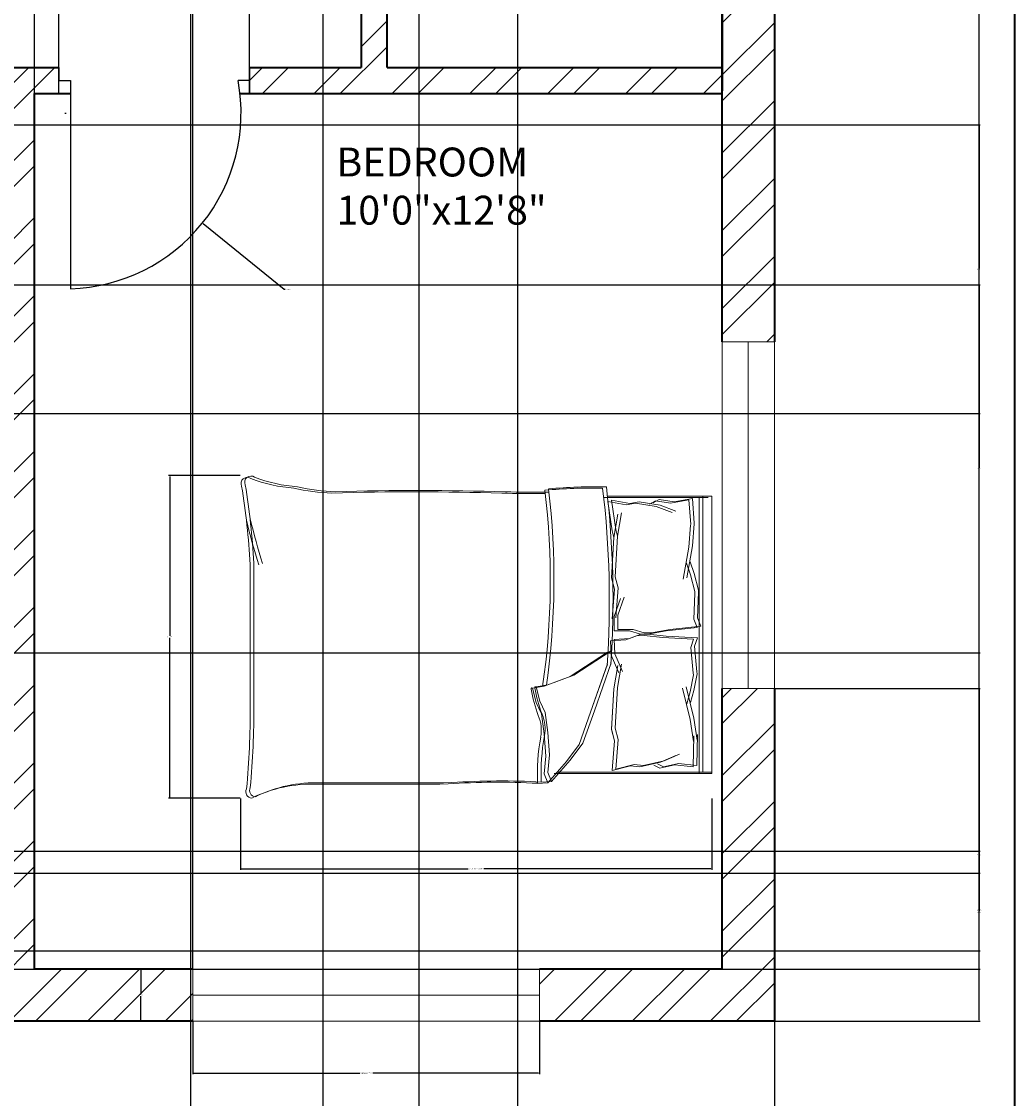
# Model space of a CAD drawing. Units: inches. Extents: x 2529 to 3014, y 1203 to 2262.
# Tile 6 of 13: x 2842 to 3014, y 1560 to 1746. Entities that reach past the tile are written whole.
import ezdxf

# ---------------------------------------------------------------- set-up
doc = ezdxf.new("R2010")
doc.units = ezdxf.units.IN
for name, color, linetype, lineweight in [('A-ANNO-DIMS', 2, 'Continuous', 18), ('A-ANNO-TTLB', 7, 'Continuous', 35), ('A-AREA-IDEN', 7, 'Continuous', 18), ('A-DOOR', 21, 'Continuous', 25), ('A-FURN', 8, 'Continuous', 18), ('A-GLAZ', 191, 'Continuous', 18), ('A-WALL', 7, 'Continuous', 35), ('A-WALL-PATT', 143, 'Continuous', 13)]:
    doc.layers.add(name, color=color, linetype=linetype, lineweight=lineweight)
doc.styles.get("Standard").update_dxf_attribs({"font": 'arial.ttf'})
doc.dimstyles.get("Standard").update_dxf_attribs({"dimtxt": 0.18, "dimasz": 0.18, "dimexe": 0.18, "dimexo": 0.0625, "dimgap": 0.09, "dimtad": 0, "dimtih": 1, "dimtoh": 1, "dimdec": 4, "dimzin": 0, "dimdsep": 46, "dimtxsty": 'Standard', "dimcen": 0.09, "dimadec": 0, "dimazin": 0, "dimtfac": 1, "dimtdec": 4, "dimtofl": 0, "dimtmove": 0, "dimatfit": 3, "dimfxl": 1, "dimtolj": 1, "dimtzin": 0, "dimarcsym": 0})

# ---------------------------------------------------------------- blocks, each defined once
blk = doc.blocks.new('BED-DOUBLE')
for p, q in [((3.48, 63.33), (3.48, 81.44)), ((3.48, 63.33), (3.48, 81.44)), ((3.48, 81.44), (51.49, 81.44)), ((3.7, 62.69), (3.7, 80.8)), ((3.7, 62.69), (3.7, 80.8)), ((51.27, 81.44), (51.27, 54.83)), ((51.27, 81.44), (51.27, 54.83)), ((51.49, 81.44), (51.49, 80.8)), ((51.49, 80.8), (51.49, 54.19)), ((51.49, 80.8), (51.49, 54.19)), ((3.48, 79.91), (51.27, 79.91)), ((3.48, 79.91), (51.27, 79.91)), ((3.7, 79.27), (51.49, 79.27)), ((3.7, 79.27), (51.49, 79.27)), ((3.9, 78.11), (8.18, 78.43)), ((3.9, 78.11), (8.18, 78.43)), ((8.18, 78.43), (8.29, 78.42)), ((8.18, 78.43), (8.29, 78.42)), ((8.29, 78.42), (12.11, 78.13)), ((8.29, 78.42), (12.11, 78.13)), ((14.86, 77.69), (16.88, 78.42)), ((14.86, 77.69), (16.88, 78.42)), ((16.88, 78.42), (19.77, 79.14)), ((16.88, 78.42), (19.77, 79.14)), ((17.11, 77.78), (20, 78.5)), ((17.11, 77.78), (20, 78.5)), ((19.77, 79.14), (20.09, 79.14)), ((19.77, 79.14), (20.09, 79.14)), ((20, 78.5), (20.32, 78.5)), ((20, 78.5), (20.32, 78.5)), ((20.09, 79.14), (24.54, 78.99)), ((20.09, 79.14), (24.54, 78.99)), ((20.32, 78.5), (24.77, 78.36)), ((20.32, 78.5), (24.77, 78.36)), ((24.54, 78.99), (25.98, 79.57)), ((24.54, 78.99), (25.98, 79.57)), ((24.77, 78.36), (26.21, 78.93)), ((24.77, 78.36), (26.21, 78.93)), ((25.98, 79.57), (26.56, 74.22)), ((25.98, 79.57), (26.56, 74.22)), ((26.21, 78.93), (26.79, 73.58)), ((26.21, 78.93), (26.79, 73.58)), ((27.98, 78.95), (27.73, 73.58)), ((27.98, 78.95), (27.73, 73.58)), ((28.21, 78.31), (27.96, 72.94)), ((28.21, 78.31), (27.96, 72.94)), ((29.46, 78.46), (27.98, 78.95)), ((29.46, 78.46), (27.98, 78.95)), ((29.68, 77.83), (28.21, 78.31)), ((29.68, 77.83), (28.21, 78.31)), ((33.88, 78.89), (29.46, 78.46)), ((33.88, 78.89), (29.46, 78.46)), ((34.21, 78.91), (33.88, 78.89)), ((34.21, 78.91), (33.88, 78.89)), ((34.43, 78.27), (34.11, 78.25)), ((34.43, 78.27), (34.11, 78.25)), ((37.14, 78.37), (34.21, 78.91)), ((37.14, 78.37), (34.21, 78.91)), ((37.36, 77.73), (34.43, 78.27)), ((37.36, 77.73), (34.43, 78.27)), ((41.91, 78.37), (36.5, 77.02)), ((41.91, 78.37), (36.5, 77.02)), ((39.2, 77.77), (37.14, 78.37)), ((39.2, 77.77), (37.14, 78.37)), ((45.71, 78.9), (41.91, 78.37)), ((45.71, 78.9), (41.91, 78.37)), ((50.11, 78.89), (44.71, 78.98)), ((44.71, 78.98), (45.71, 78.9)), ((50.11, 78.89), (44.71, 78.98)), ((44.71, 78.98), (45.71, 78.9)), ((50.34, 78.25), (44.94, 78.34)), ((44.94, 78.34), (45.94, 78.26)), ((50.34, 78.25), (44.94, 78.34)), ((44.94, 78.34), (45.94, 78.26)), ((50.11, 78.89), (49.73, 75.68)), ((50.11, 78.89), (49.73, 75.68)), ((3.9, 78.13), (4.47, 74.95)), ((3.9, 78.13), (4.47, 74.95)), ((4.12, 77.49), (4.7, 74.31)), ((4.12, 77.49), (4.7, 74.31)), ((4.13, 77.47), (8.41, 77.8)), ((4.13, 77.47), (8.41, 77.8)), ((8.41, 77.8), (8.51, 77.78)), ((8.41, 77.8), (8.51, 77.78)), ((8.51, 77.78), (12.34, 77.49)), ((8.51, 77.78), (12.34, 77.49)), ((12.11, 78.13), (17.6, 77.12)), ((12.11, 78.13), (17.6, 77.12)), ((12.34, 77.49), (17.83, 76.48)), ((12.34, 77.49), (17.83, 76.48)), ((15.08, 77.05), (17.11, 77.78)), ((15.08, 77.05), (17.11, 77.78)), ((34.11, 78.25), (29.68, 77.83)), ((34.11, 78.25), (29.68, 77.83)), ((42.14, 77.73), (36.72, 76.38)), ((42.14, 77.73), (36.72, 76.38)), ((39.43, 77.13), (37.36, 77.73)), ((39.43, 77.13), (37.36, 77.73)), ((45.94, 78.26), (42.14, 77.73)), ((45.94, 78.26), (42.14, 77.73)), ((50.34, 78.25), (49.96, 75.04)), ((50.34, 78.25), (49.96, 75.04)), ((4.47, 74.95), (4.04, 72.34)), ((4.47, 74.95), (4.04, 72.34)), ((5.05, 72.49), (6.06, 75.24)), ((5.05, 72.49), (6.06, 75.24)), ((5.28, 71.85), (6.29, 74.6)), ((5.28, 71.85), (6.29, 74.6)), ((49.31, 73.19), (48.13, 75.87)), ((49.31, 73.19), (48.13, 75.87)), ((49.54, 72.55), (48.36, 75.23)), ((49.54, 72.55), (48.36, 75.23)), ((49.73, 75.68), (50.33, 73.11)), ((49.73, 75.68), (50.33, 73.11)), ((49.96, 75.04), (50.56, 72.47)), ((49.96, 75.04), (50.56, 72.47)), ((4.7, 74.31), (4.27, 71.7)), ((4.7, 74.31), (4.27, 71.7)), ((26.56, 74.22), (27.14, 71.04)), ((26.56, 74.22), (27.14, 71.04)), ((26.79, 73.58), (27.37, 70.4)), ((26.79, 73.58), (27.37, 70.4)), ((27.73, 73.58), (27.36, 70.37)), ((27.73, 73.58), (27.36, 70.37)), ((27.96, 72.94), (27.58, 69.73)), ((27.96, 72.94), (27.58, 69.73)), ((50.11, 69.61), (49.31, 73.19)), ((50.11, 69.61), (49.31, 73.19)), ((50.33, 73.11), (49.81, 72.06)), ((50.33, 73.11), (49.82, 72.06)), ((4.04, 72.34), (4.62, 71.33)), ((4.04, 72.34), (4.62, 71.33)), ((4.27, 71.7), (4.85, 70.69)), ((4.27, 71.7), (4.85, 70.69)), ((4.47, 68.87), (5.05, 72.49)), ((4.47, 68.87), (5.05, 72.49)), ((4.7, 68.23), (5.28, 71.85)), ((4.7, 68.23), (5.28, 71.85)), ((27.14, 71.04), (27.14, 69.74)), ((27.14, 71.04), (27.14, 69.74)), ((50.34, 68.98), (49.54, 72.55)), ((50.34, 68.98), (49.54, 72.55)), ((50.56, 72.47), (50.04, 71.42)), ((50.56, 72.47), (50.04, 71.42)), ((27.14, 69.74), (26.56, 67.86)), ((27.14, 69.74), (26.56, 67.86)), ((27.37, 69.1), (26.79, 67.22)), ((27.37, 69.1), (26.79, 67.22)), ((27.36, 70.37), (27.44, 69.07)), ((27.36, 70.37), (27.44, 69.07)), ((27.37, 70.4), (27.37, 69.1)), ((27.37, 70.4), (27.37, 69.1)), ((27.44, 69.07), (28.13, 67.23)), ((27.44, 69.07), (28.13, 67.23)), ((27.58, 69.73), (27.67, 68.43)), ((27.58, 69.73), (27.66, 68.43)), ((49.92, 68.01), (50.11, 69.61)), ((49.92, 68.01), (50.11, 69.61)), ((50.15, 67.37), (50.34, 68.98)), ((50.15, 67.37), (50.34, 68.98)), ((4.18, 64.1), (4.76, 67.28)), ((4.18, 64.1), (4.76, 67.28)), ((4.76, 67.28), (4.47, 68.87)), ((4.76, 67.28), (4.47, 68.87)), ((4.99, 66.64), (4.7, 68.23)), ((4.99, 66.64), (4.7, 68.23)), ((26.56, 67.86), (26.56, 65.18)), ((26.56, 67.86), (26.56, 65.18)), ((26.79, 67.22), (26.79, 64.54)), ((26.79, 67.22), (26.79, 64.54)), ((27.66, 68.43), (28.36, 66.59)), ((27.67, 68.43), (28.36, 66.59)), ((28.13, 67.23), (28.3, 64.55)), ((28.13, 67.23), (28.3, 64.55)), ((50.7, 64.87), (49.92, 68.01)), ((50.7, 64.87), (49.92, 68.01)), ((50.93, 64.23), (50.15, 67.37)), ((50.93, 64.23), (50.15, 67.37)), ((4.41, 63.46), (4.99, 66.64)), ((4.41, 63.46), (4.99, 66.64)), ((6.38, 65.81), (10.41, 65.15)), ((6.38, 65.81), (10.41, 65.15)), ((17.42, 64.72), (19.38, 65.27)), ((17.42, 64.72), (19.38, 65.27)), ((19.38, 65.27), (24.52, 64.87)), ((19.38, 65.27), (24.52, 64.87)), ((24.1, 65.18), (20.96, 66.27)), ((24.1, 65.18), (20.96, 66.27)), ((24.33, 64.54), (21.19, 65.63)), ((24.33, 64.54), (21.19, 65.63)), ((28.36, 66.59), (28.53, 63.91)), ((28.36, 66.59), (28.53, 63.91)), ((30.75, 64.7), (33.82, 65.99)), ((30.75, 64.7), (33.82, 65.99)), ((30.98, 64.06), (34.05, 65.35)), ((30.98, 64.06), (34.05, 65.35)), ((32.56, 65.81), (36.6, 65.15)), ((32.56, 65.81), (36.6, 65.15)), ((43.61, 64.72), (45.57, 65.27)), ((43.61, 64.72), (45.57, 65.27)), ((45.57, 65.27), (50.7, 64.87)), ((45.57, 65.27), (50.7, 64.87)), ((9.28, 64.83), (4.18, 64.1)), ((9.28, 64.83), (4.18, 64.1)), ((9.51, 64.19), (4.41, 63.46)), ((9.51, 64.19), (4.41, 63.46)), ((6.61, 65.18), (10.64, 64.51)), ((6.61, 65.18), (10.64, 64.51)), ((10.41, 65.15), (9.28, 64.83)), ((10.41, 65.15), (9.28, 64.83)), ((10.64, 64.51), (9.51, 64.19)), ((10.64, 64.51), (9.51, 64.19)), ((10.41, 65.15), (17.42, 64.72)), ((10.41, 65.15), (17.42, 64.72)), ((10.64, 64.51), (17.65, 64.08)), ((10.64, 64.51), (17.65, 64.08)), ((17.65, 64.08), (19.61, 64.64)), ((17.65, 64.08), (19.61, 64.64)), ((19.61, 64.64), (24.74, 64.23)), ((19.61, 64.64), (24.74, 64.23)), ((26.56, 65.18), (24.1, 65.18)), ((26.56, 65.18), (24.1, 65.18)), ((26.79, 64.54), (24.33, 64.54)), ((26.79, 64.54), (24.33, 64.54)), ((28.3, 64.55), (30.75, 64.7)), ((28.3, 64.55), (30.75, 64.7)), ((28.53, 63.91), (30.98, 64.06)), ((28.53, 63.91), (30.98, 64.06)), ((30.26, 64.06), (34.45, 57.57)), ((30.26, 64.06), (34.45, 57.57)), ((30.49, 63.42), (34.68, 56.93)), ((30.49, 63.42), (34.68, 56.93)), ((40.64, 61.13), (32.31, 64.06)), ((40.64, 61.13), (32.31, 64.06)), ((40.87, 60.49), (32.53, 63.42)), ((40.87, 60.49), (32.54, 63.42)), ((32.79, 65.18), (36.83, 64.51)), ((32.79, 65.18), (36.82, 64.51)), ((36.6, 65.15), (43.61, 64.72)), ((36.6, 65.15), (43.61, 64.72)), ((36.82, 64.51), (43.83, 64.08)), ((36.83, 64.51), (43.84, 64.08)), ((43.83, 64.08), (45.8, 64.64)), ((43.84, 64.08), (45.8, 64.64)), ((45.8, 64.64), (50.93, 64.23)), ((45.8, 64.64), (50.93, 64.23)), ((46.22, 59.11), (40.64, 61.13)), ((46.22, 59.11), (40.64, 61.13)), ((46.45, 58.48), (40.87, 60.49)), ((46.45, 58.48), (40.87, 60.49)), ((49.16, 56.95), (46.22, 59.11)), ((49.16, 56.95), (46.22, 59.11)), ((49.39, 56.31), (46.45, 58.48)), ((49.39, 56.31), (46.45, 58.48)), ((34.45, 57.57), (36.15, 53.08)), ((34.45, 57.57), (36.15, 53.08)), ((34.68, 56.93), (36.38, 52.44)), ((34.68, 56.93), (36.38, 52.44)), ((52.87, 53.7), (49.16, 56.95)), ((52.87, 53.7), (49.16, 56.95)), ((53.1, 53.06), (49.39, 56.31)), ((53.1, 53.06), (49.39, 56.31)), ((36.15, 53.08), (36.46, 51.07)), ((36.15, 53.08), (36.46, 51.07)), ((36.38, 52.44), (36.69, 50.43)), ((36.38, 52.44), (36.69, 50.43)), ((38.94, 51.69), (40.95, 52.61)), ((38.94, 51.69), (40.95, 52.61)), ((40.95, 52.61), (44.36, 53.08)), ((40.95, 52.61), (44.36, 53.08)), ((41.18, 51.97), (44.59, 52.44)), ((41.18, 51.97), (44.59, 52.44)), ((44.36, 53.08), (48.23, 53.39)), ((44.36, 53.08), (48.23, 53.39)), ((44.59, 52.44), (48.46, 52.75)), ((44.59, 52.44), (48.46, 52.75)), ((48.23, 53.39), (51.33, 53.08)), ((48.23, 53.39), (51.33, 53.08)), ((48.46, 52.75), (51.56, 52.44)), ((48.46, 52.75), (51.56, 52.44)), ((51.33, 53.08), (52.87, 53.7)), ((51.33, 53.08), (52.87, 53.7)), ((51.56, 52.44), (53.1, 53.06)), ((51.56, 52.44), (53.1, 53.06)), ((52.95, 51.95), (52.87, 53.7, 3.87)), ((52.95, 51.95), (52.87, 53.7, 3.87)), ((53.18, 51.31), (53.1, 53.06, 3.87)), ((53.18, 51.31), (53.1, 53.06, 3.87)), ((36.46, 51.07), (38.94, 51.69)), ((36.46, 51.07), (38.94, 51.69)), ((36.69, 50.43), (39.17, 51.05)), ((36.69, 50.43), (39.17, 51.05)), ((39.17, 51.05), (41.18, 51.97)), ((39.17, 51.05), (41.18, 51.97)), ((15.06, 2.2), (39.68, 2.2)), ((15.06, 2.2), (39.68, 2.2)), ((15.29, 1.56), (39.91, 1.56)), ((15.29, 1.56), (39.91, 1.56))]:
    blk.add_line(p, q)
for centre, radius, start, end in [((21.36, -100.61), 164.97, 86.0865, 96.7821), ((21.36, -100.61), 164.97, 86.0865, 96.7821), ((21.59, -101.25), 164.97, 86.0865, 96.7821), ((21.59, -101.25), 164.97, 86.0865, 96.7821), ((85.16, 61.35), 83.31, 178.7218, 185.604), ((85.16, 61.35), 83.31, 178.7218, 185.604), ((85.39, 60.71), 83.31, 178.7218, 185.604), ((85.39, 60.71), 83.31, 178.7218, 185.604), ((17.76, -74.87), 129.02, 81.7845, 96.9006), ((17.76, -74.87), 129.02, 81.7845, 96.9006), ((17.98, -75.51), 129.02, 81.7845, 96.9006), ((17.98, -75.51), 129.02, 81.7845, 96.9006), ((-167.31, 50.27), 170.11, 358.4762, 1.0082), ((-167.31, 50.27), 170.11, 358.4762, 1.0082), ((-167.08, 49.63), 170.11, 358.4762, 1.0082), ((-167.08, 49.63), 170.11, 358.4762, 1.0082), ((43.74, 46.38), 6.22, 78.6608, 113.7384), ((43.74, 46.38), 6.22, 78.6608, 113.7384), ((51.33, 88.1), 36.18, 259.8763, 272.5657), ((51.33, 88.1), 36.18, 259.8763, 272.5657), ((36.64, 51), 0.185, 160.2464, 271.1377), ((36.64, 51), 0.185, 160.2464, 271.1377), ((31.15, 79.96), 29.65, 280.6617, 289.8806), ((31.15, 79.96), 29.65, 280.6617, 289.8806), ((36.87, 50.36), 0.185, 160.2464, 271.1377), ((36.86, 50.36), 0.185, 160.2464, 271.1377), ((31.38, 79.32), 29.65, 280.6617, 289.8806), ((31.38, 79.32), 29.65, 280.6617, 289.8806), ((43.97, 45.74), 6.22, 78.6608, 113.7384), ((43.97, 45.74), 6.22, 78.6608, 113.7384), ((51.56, 87.46), 36.18, 259.8763, 272.5657), ((51.56, 87.46), 36.18, 259.8763, 272.5657), ((182.27, 45.13), 129.5, 176.9791, 183.8365), ((182.27, 45.13), 129.5, 176.9791, 183.8365), ((182.49, 44.49), 129.5, 176.9791, 183.8365), ((182.49, 44.49), 129.5, 176.9791, 183.8365), ((484.82, 30.83), 482.31, 178.2277, 181.7185), ((484.82, 30.83), 482.31, 178.2277, 181.7185), ((485.05, 30.19), 482.31, 178.2277, 181.7185), ((485.05, 30.19), 482.31, 178.2277, 181.7185), ((-4508.74, 13.62), 4561.86, 0.00217, 0.28689), ((-4508.74, 13.62), 4561.86, 0.00217, 0.28689), ((-4508.51, 12.98), 4561.86, 0.00217, 0.28689), ((-4508.51, 12.98), 4561.86, 0.00217, 0.28689), ((-26.9, 16.93), 29.63, 346.0648, 358.9113), ((-26.9, 16.93), 29.63, 346.0648, 358.9113), ((-26.67, 16.29), 29.63, 346.0648, 358.9113), ((-26.67, 16.29), 29.63, 346.0648, 358.9113), ((76.16, 12.78), 23.07, 177.4714, 206.4681), ((76.16, 12.78), 23.07, 177.4714, 206.4681), ((76.39, 12.14), 23.07, 177.4714, 206.4681), ((76.39, 12.14), 23.07, 177.4714, 206.4681), ((-21.66, 11.17), 23.56, 337.9751, 356.652), ((-21.66, 11.17), 23.56, 337.9751, 356.652), ((-21.43, 10.53), 23.56, 337.9751, 356.652), ((-21.43, 10.53), 23.56, 337.9751, 356.652), ((-17.22, 105.16), 106.46, 283.3832, 287.7053), ((-17.22, 105.16), 106.46, 283.3832, 287.7053), ((1.09, 1.73), 1.09, 146.1736, 293.4781), ((1.09, 1.73), 1.09, 146.1736, 293.4781), ((21.43, -119.39), 121.76, 92.9958, 99.4091), ((21.43, -119.39), 121.76, 92.9958, 99.4091), ((-16.99, 104.52), 106.46, 283.3832, 287.7053), ((-16.99, 104.52), 106.46, 283.3832, 287.7053), ((41.15, -130.83), 133.04, 84.4998, 90.6351), ((41.15, -130.83), 133.04, 84.4998, 90.6351), ((54.41, 2.57), 1.1, 242.6588, 356.02), ((54.41, 2.57), 1.1, 242.6588, 356.02), ((1.32, 1.09), 1.09, 146.1736, 293.4781), ((1.32, 1.09), 1.09, 146.1736, 293.4781), ((21.66, -120.03), 121.76, 92.9958, 99.4091), ((21.66, -120.03), 121.76, 92.9958, 99.4091), ((41.38, -131.47), 133.04, 84.4998, 90.6351), ((41.38, -131.47), 133.04, 84.4998, 90.6351), ((54.64, 1.93), 1.1, 242.6588, 356.02), ((54.64, 1.93), 1.1, 242.6588, 356.02)]:
    blk.add_arc(centre, radius, start, end)
blk = doc.blocks.new('WIN-60x9')
for p, q in [((0, 60), (9, 60)), ((0, 60), (0, 0)), ((9, 60), (4.5, 60)), ((4.5, 60), (4.5, 0)), ((9, 60), (9, 0)), ((4.5, 0), (0, 0)), ((0, 0), (9, 0))]:
    blk.add_line(p, q)
blk = doc.blocks.new('*D6')
at = {"layer": 'A-ANNO-DIMS', "color": 0, "lineweight": -2, "transparency": 16777216}
for p, q in [((2871.44, 1573.44), (2871.44, 1564.32)), ((2931.44, 1573.44), (2931.44, 1564.32)), ((2871.62, 1564.5), (2900.32, 1564.5)), ((2931.26, 1564.5), (2902.56, 1564.5))]:
    blk.add_line(p, q, dxfattribs=at)
at = {"layer": 'A-ANNO-DIMS', "color": 0, "transparency": 16777216}
for points in [[(2871.62, 1564.53), (2871.62, 1564.47), (2871.44, 1564.5)], [(2931.26, 1564.53), (2931.26, 1564.47), (2931.44, 1564.5)]]:
    blk.add_solid(points, dxfattribs=at)
at = {"layer": 'Defpoints', "color": 0, "transparency": 16777216}
for p in [(2871.44, 1573.5), (2931.44, 1573.5), (2871.44, 1564.5)]:
    blk.add_point(p, dxfattribs=at)
at = {"layer": 'A-ANNO-DIMS', "color": 0, "transparency": 16777216, "insert": (2901.44, 1564.5), "char_height": 0.18, "attachment_point": 5}
blk.add_mtext('\\A1;WINDOW 60 TYP.', dxfattribs=at)
blk = doc.blocks.new('*D7')
at = {"layer": 'A-ANNO-DIMS', "color": 0, "lineweight": -2, "transparency": 16777216}
for p, q in [((2871.38, 1582.5), (2862.26, 1582.5)), ((2862.44, 1582.32), (2862.44, 1578.19)), ((2862.44, 1573.68), (2862.44, 1577.82)), ((2871.38, 1573.5), (2862.26, 1573.5))]:
    blk.add_line(p, q, dxfattribs=at)
at = {"layer": 'A-ANNO-DIMS', "color": 0, "transparency": 16777216}
for points in [[(2862.41, 1582.32), (2862.47, 1582.32), (2862.44, 1582.5)], [(2862.41, 1573.68), (2862.47, 1573.68), (2862.44, 1573.5)]]:
    blk.add_solid(points, dxfattribs=at)
at = {"layer": 'Defpoints', "color": 0, "transparency": 16777216}
for p in [(2862.44, 1582.5), (2871.44, 1582.5), (2871.44, 1573.5)]:
    blk.add_point(p, dxfattribs=at)
at = {"layer": 'A-ANNO-DIMS', "color": 0, "transparency": 16777216, "insert": (2862.44, 1578), "char_height": 0.18, "attachment_point": 5}
blk.add_mtext('\\A1;9 TYP.', dxfattribs=at)
blk = doc.blocks.new('*D10')
at = {"layer": 'A-ANNO-DIMS', "color": 0, "lineweight": -2, "transparency": 16777216}
for p, q in [((2879.68, 1612.04), (2879.68, 1599.69)), ((2961.23, 1612.04), (2961.23, 1599.69)), ((2879.86, 1599.87), (2919.08, 1599.87)), ((2961.05, 1599.87), (2921.82, 1599.87))]:
    blk.add_line(p, q, dxfattribs=at)
at = {"layer": 'A-ANNO-DIMS', "color": 0, "transparency": 16777216}
for points in [[(2879.86, 1599.9), (2879.86, 1599.84), (2879.68, 1599.87)], [(2961.05, 1599.9), (2961.05, 1599.84), (2961.23, 1599.87)]]:
    blk.add_solid(points, dxfattribs=at)
at = {"layer": 'Defpoints', "color": 0, "transparency": 16777216}
for p in [(2879.68, 1612.11), (2961.23, 1612.11), (2961.23, 1599.87)]:
    blk.add_point(p, dxfattribs=at)
at = {"layer": 'A-ANNO-DIMS', "color": 0, "transparency": 16777216, "insert": (2920.45, 1599.87), "char_height": 0.18, "attachment_point": 5}
blk.add_mtext('\\A1;DOUBLE BED 82 TYP.', dxfattribs=at)
blk = doc.blocks.new('*D11')
at = {"layer": 'A-ANNO-DIMS', "color": 0, "lineweight": -2, "transparency": 16777216}
for p, q in [((2879.61, 1667.93), (2867.26, 1667.93)), ((2867.44, 1667.75), (2867.44, 1640.2)), ((2867.44, 1612.29), (2867.44, 1639.84)), ((2879.61, 1612.11), (2867.26, 1612.11))]:
    blk.add_line(p, q, dxfattribs=at)
at = {"layer": 'A-ANNO-DIMS', "color": 0, "transparency": 16777216}
for points in [[(2867.41, 1667.75), (2867.47, 1667.75), (2867.44, 1667.93)], [(2867.41, 1612.29), (2867.47, 1612.29), (2867.44, 1612.11)]]:
    blk.add_solid(points, dxfattribs=at)
at = {"layer": 'Defpoints', "color": 0, "transparency": 16777216}
for p in [(2879.68, 1667.93), (2867.44, 1612.11), (2879.68, 1612.11)]:
    blk.add_point(p, dxfattribs=at)
at = {"layer": 'A-ANNO-DIMS', "color": 0, "transparency": 16777216, "insert": (2867.44, 1640.02), "char_height": 0.18, "attachment_point": 5}
blk.add_mtext('\\A1;56 TYP.', dxfattribs=at)
blk = doc.blocks.new('*D17')
at = {"layer": 'A-ANNO-DIMS', "color": 0, "lineweight": -2, "transparency": 16777216}
for p, q in [((2972.12, 2207.5), (3007.66, 2207.5)), ((3007.48, 2207.32), (3007.48, 1890.69)), ((3007.48, 1573.68), (3007.48, 1890.32)), ((2972.12, 1573.5), (3007.66, 1573.5))]:
    blk.add_line(p, q, dxfattribs=at)
at = {"layer": 'A-ANNO-DIMS', "color": 0, "transparency": 16777216}
for points in [[(3007.45, 2207.32), (3007.51, 2207.32), (3007.48, 2207.5)], [(3007.45, 1573.68), (3007.51, 1573.68), (3007.48, 1573.5)]]:
    blk.add_solid(points, dxfattribs=at)
at = {"layer": 'Defpoints', "color": 0, "transparency": 16777216}
for p in [(2972.06, 2207.5), (3007.48, 2207.5), (2972.06, 1573.5)]:
    blk.add_point(p, dxfattribs=at)
at = {"layer": 'A-ANNO-DIMS', "color": 0, "transparency": 16777216, "insert": (3007.48, 1890.5), "char_height": 0.18, "attachment_point": 5}
blk.add_mtext('\\A1;634', dxfattribs=at)
blk = doc.blocks.new('*D20')
at = {"layer": 'A-ANNO-DIMS', "color": 0, "lineweight": -2, "transparency": 16777216}
for p, q in [((2839.56, 1582.44), (2839.56, 1483.77)), ((2972.06, 1573.44), (2972.06, 1483.77)), ((2839.74, 1483.95), (2905.42, 1483.95)), ((2971.88, 1483.95), (2906.19, 1483.95))]:
    blk.add_line(p, q, dxfattribs=at)
at = {"layer": 'A-ANNO-DIMS', "color": 0, "transparency": 16777216}
for points in [[(2839.74, 1483.98), (2839.74, 1483.92), (2839.56, 1483.95)], [(2971.88, 1483.98), (2971.88, 1483.92), (2972.06, 1483.95)]]:
    blk.add_solid(points, dxfattribs=at)
at = {"layer": 'Defpoints', "color": 0, "transparency": 16777216}
for p in [(2839.56, 1582.5), (2972.06, 1573.5), (2972.06, 1483.95)]:
    blk.add_point(p, dxfattribs=at)
at = {"layer": 'A-ANNO-DIMS', "color": 0, "transparency": 16777216, "insert": (2905.81, 1483.95), "char_height": 0.18, "attachment_point": 5}
blk.add_mtext('\\A1;132.5', dxfattribs=at)
blk = doc.blocks.new('*D38')
at = {"layer": 'A-ANNO-DIMS', "color": 0, "lineweight": -2, "transparency": 16777216}
for p, q in [((2844.06, 1582.57), (2844.06, 2243.11)), ((2844.24, 2242.93), (2857.35, 2242.93)), ((2871.26, 2242.93), (2858.14, 2242.93)), ((2871.44, 1582.57), (2871.44, 2243.11))]:
    blk.add_line(p, q, dxfattribs=at)
at = {"layer": 'A-ANNO-DIMS', "color": 0, "transparency": 16777216}
for points in [[(2844.24, 2242.96), (2844.24, 2242.9), (2844.06, 2242.93)], [(2871.26, 2242.96), (2871.26, 2242.9), (2871.44, 2242.93)]]:
    blk.add_solid(points, dxfattribs=at)
at = {"layer": 'Defpoints', "color": 0, "transparency": 16777216}
for p in [(2871.44, 2242.93), (2844.06, 1582.5), (2871.44, 1582.5)]:
    blk.add_point(p, dxfattribs=at)
at = {"layer": 'A-ANNO-DIMS', "color": 0, "transparency": 16777216, "insert": (2857.75, 2242.93), "char_height": 0.18, "attachment_point": 5}
blk.add_mtext('\\A1;27.39', dxfattribs=at)
blk = doc.blocks.new('*D39')
at = {"layer": 'A-ANNO-DIMS', "color": 0, "lineweight": -2, "transparency": 16777216}
for p, q in [((2848.27, 1734.07), (2848.27, 2243.11)), ((2848.45, 2242.93), (2864.3, 2242.93)), ((2881.08, 2242.93), (2865.23, 2242.93)), ((2881.26, 1734.07), (2881.26, 2243.11))]:
    blk.add_line(p, q, dxfattribs=at)
at = {"layer": 'A-ANNO-DIMS', "color": 0, "transparency": 16777216}
for points in [[(2848.45, 2242.96), (2848.45, 2242.9), (2848.27, 2242.93)], [(2881.08, 2242.96), (2881.08, 2242.9), (2881.26, 2242.93)]]:
    blk.add_solid(points, dxfattribs=at)
at = {"layer": 'Defpoints', "color": 0, "transparency": 16777216}
for p in [(2881.26, 2242.93), (2848.27, 1734), (2881.26, 1734)]:
    blk.add_point(p, dxfattribs=at)
at = {"layer": 'A-ANNO-DIMS', "color": 0, "transparency": 16777216, "insert": (2864.76, 2242.93), "char_height": 0.18, "attachment_point": 5}
blk.add_mtext('\\A1;32.994', dxfattribs=at)
blk = doc.blocks.new('*D43')
at = {"layer": 'A-ANNO-DIMS', "color": 0, "lineweight": -2, "transparency": 16777216}
for p, q in [((2616.77, 1700.93), (3007.66, 1700.93)), ((3007.48, 1700.75), (3007.48, 1669.26)), ((3007.48, 1637.41), (3007.48, 1668.9)), ((2616.77, 1637.23), (3007.66, 1637.23))]:
    blk.add_line(p, q, dxfattribs=at)
at = {"layer": 'A-ANNO-DIMS', "color": 0, "transparency": 16777216}
for points in [[(3007.45, 1700.75), (3007.51, 1700.75), (3007.48, 1700.93)], [(3007.45, 1637.41), (3007.51, 1637.41), (3007.48, 1637.23)]]:
    blk.add_solid(points, dxfattribs=at)
at = {"layer": 'Defpoints', "color": 0, "transparency": 16777216}
for p in [(2616.71, 1700.93), (3007.48, 1700.93), (2616.71, 1637.23)]:
    blk.add_point(p, dxfattribs=at)
at = {"layer": 'A-ANNO-DIMS', "color": 0, "transparency": 16777216, "insert": (3007.48, 1669.08), "char_height": 0.18, "attachment_point": 5}
blk.add_mtext('\\A1;63.7', dxfattribs=at)
blk = doc.blocks.new('*D45')
at = {"layer": 'A-ANNO-DIMS', "color": 0, "lineweight": -2, "transparency": 16777216}
for p, q in [((2655.95, 1728.6), (3007.66, 1728.6)), ((3007.48, 1728.42), (3007.48, 1703.82)), ((3007.48, 1678.86), (3007.48, 1703.46)), ((2655.95, 1678.68), (3007.66, 1678.68))]:
    blk.add_line(p, q, dxfattribs=at)
at = {"layer": 'A-ANNO-DIMS', "color": 0, "transparency": 16777216}
for points in [[(3007.45, 1728.42), (3007.51, 1728.42), (3007.48, 1728.6)], [(3007.45, 1678.86), (3007.51, 1678.86), (3007.48, 1678.68)]]:
    blk.add_solid(points, dxfattribs=at)
at = {"layer": 'Defpoints', "color": 0, "transparency": 16777216}
for p in [(2655.89, 1728.6), (3007.48, 1728.6), (2655.89, 1678.68)]:
    blk.add_point(p, dxfattribs=at)
at = {"layer": 'A-ANNO-DIMS', "color": 0, "transparency": 16777216, "insert": (3007.48, 1703.64), "char_height": 0.18, "attachment_point": 5}
blk.add_mtext('\\A1;49.92', dxfattribs=at)
blk = doc.blocks.new('*D51')
at = {"layer": 'A-ANNO-DIMS', "color": 0, "lineweight": -2, "transparency": 16777216}
for p, q in [((2972.12, 1631.08), (3007.66, 1631.08)), ((3007.48, 1630.9), (3007.48, 1602.47)), ((3007.48, 1573.68), (3007.48, 1602.11)), ((2972.12, 1573.5), (3007.66, 1573.5))]:
    blk.add_line(p, q, dxfattribs=at)
at = {"layer": 'A-ANNO-DIMS', "color": 0, "transparency": 16777216}
for points in [[(3007.45, 1630.9), (3007.51, 1630.9), (3007.48, 1631.08)], [(3007.45, 1573.68), (3007.51, 1573.68), (3007.48, 1573.5)]]:
    blk.add_solid(points, dxfattribs=at)
at = {"layer": 'Defpoints', "color": 0, "transparency": 16777216}
for p in [(2972.06, 1631.08), (3007.48, 1631.08), (2972.06, 1573.5)]:
    blk.add_point(p, dxfattribs=at)
at = {"layer": 'A-ANNO-DIMS', "color": 0, "transparency": 16777216, "insert": (3007.48, 1602.29), "char_height": 0.18, "attachment_point": 5}
blk.add_mtext('\\A1;57.57', dxfattribs=at)
blk = doc.blocks.new('*D57')
at = {"layer": 'A-ANNO-DIMS', "color": 0, "lineweight": -2, "transparency": 16777216}
for p, q in [((2871.06, 2198.44), (2871.06, 1483.77)), ((2893.92, 2198.44), (2893.92, 1483.77)), ((2871.24, 1483.95), (2882.02, 1483.95)), ((2893.74, 1483.95), (2882.95, 1483.95))]:
    blk.add_line(p, q, dxfattribs=at)
at = {"layer": 'A-ANNO-DIMS', "color": 0, "transparency": 16777216}
for points in [[(2871.24, 1483.98), (2871.24, 1483.92), (2871.06, 1483.95)], [(2893.74, 1483.98), (2893.74, 1483.92), (2893.92, 1483.95)]]:
    blk.add_solid(points, dxfattribs=at)
at = {"layer": 'Defpoints', "color": 0, "transparency": 16777216}
for p in [(2871.06, 2198.5), (2893.92, 2198.5), (2893.92, 1483.95)]:
    blk.add_point(p, dxfattribs=at)
at = {"layer": 'A-ANNO-DIMS', "color": 0, "transparency": 16777216, "insert": (2882.49, 1483.95), "char_height": 0.18, "attachment_point": 5}
blk.add_mtext('\\A1;22.866', dxfattribs=at)
blk = doc.blocks.new('*D75')
at = {"layer": 'A-ANNO-DIMS', "color": 0, "lineweight": -2, "transparency": 16777216}
for p, q in [((2910.52, 2189.17), (2910.52, 1483.77)), ((2893.92, 2187.06), (2893.92, 1483.77)), ((2894.1, 1483.95), (2901.91, 1483.95)), ((2910.34, 1483.95), (2902.54, 1483.95))]:
    blk.add_line(p, q, dxfattribs=at)
at = {"layer": 'A-ANNO-DIMS', "color": 0, "transparency": 16777216}
for points in [[(2894.1, 1483.98), (2894.1, 1483.92), (2893.92, 1483.95)], [(2910.34, 1483.98), (2910.34, 1483.92), (2910.52, 1483.95)]]:
    blk.add_solid(points, dxfattribs=at)
at = {"layer": 'Defpoints', "color": 0, "transparency": 16777216}
for p in [(2910.52, 2189.24), (2893.92, 2187.12), (2910.52, 1483.95)]:
    blk.add_point(p, dxfattribs=at)
at = {"layer": 'A-ANNO-DIMS', "color": 0, "transparency": 16777216, "insert": (2902.22, 1483.95), "char_height": 0.18, "attachment_point": 5}
blk.add_mtext('\\A1;16.6', dxfattribs=at)
blk = doc.blocks.new('*D76')
at = {"layer": 'A-ANNO-DIMS', "color": 0, "lineweight": -2, "transparency": 16777216}
for p, q in [((2910.52, 2189.17), (2910.52, 1483.77)), ((2927.64, 2189.17), (2927.64, 1483.77)), ((2910.7, 1483.95), (2918.63, 1483.95)), ((2927.46, 1483.95), (2919.54, 1483.95))]:
    blk.add_line(p, q, dxfattribs=at)
at = {"layer": 'A-ANNO-DIMS', "color": 0, "transparency": 16777216}
for points in [[(2910.7, 1483.98), (2910.7, 1483.92), (2910.52, 1483.95)], [(2927.46, 1483.98), (2927.46, 1483.92), (2927.64, 1483.95)]]:
    blk.add_solid(points, dxfattribs=at)
at = {"layer": 'Defpoints', "color": 0, "transparency": 16777216}
for p in [(2910.52, 2189.24), (2927.64, 2189.24), (2927.64, 1483.95)]:
    blk.add_point(p, dxfattribs=at)
at = {"layer": 'A-ANNO-DIMS', "color": 0, "transparency": 16777216, "insert": (2919.08, 1483.95), "char_height": 0.18, "attachment_point": 5}
blk.add_mtext('\\A1;17.123', dxfattribs=at)
blk = doc.blocks.new('*D79')
at = {"layer": 'A-ANNO-DIMS', "color": 0, "lineweight": -2, "transparency": 16777216}
for p, q in [((2790.78, 1599.1), (3007.66, 1599.1)), ((3007.48, 1598.92), (3007.48, 1592.58)), ((3007.48, 1585.88), (3007.48, 1592.22)), ((2790.78, 1585.7), (3007.66, 1585.7))]:
    blk.add_line(p, q, dxfattribs=at)
at = {"layer": 'A-ANNO-DIMS', "color": 0, "transparency": 16777216}
for points in [[(3007.45, 1598.92), (3007.51, 1598.92), (3007.48, 1599.1)], [(3007.45, 1585.88), (3007.51, 1585.88), (3007.48, 1585.7)]]:
    blk.add_solid(points, dxfattribs=at)
at = {"layer": 'Defpoints', "color": 0, "transparency": 16777216}
for p in [(2790.72, 1599.1), (3007.48, 1599.1), (2790.72, 1585.7)]:
    blk.add_point(p, dxfattribs=at)
at = {"layer": 'A-ANNO-DIMS', "color": 0, "transparency": 16777216, "insert": (3007.48, 1592.4), "char_height": 0.18, "attachment_point": 5}
blk.add_mtext('\\A1;13.397', dxfattribs=at)
blk = doc.blocks.new('*D80')
at = {"layer": 'A-ANNO-DIMS', "color": 0, "lineweight": -2, "transparency": 16777216}
for p, q in [((2737.62, 1602.91), (3007.66, 1602.91)), ((3007.48, 1602.73), (3007.48, 1592.89)), ((3007.48, 1582.68), (3007.48, 1592.52)), ((2737.62, 1582.5), (3007.66, 1582.5))]:
    blk.add_line(p, q, dxfattribs=at)
at = {"layer": 'A-ANNO-DIMS', "color": 0, "transparency": 16777216}
for points in [[(3007.45, 1602.73), (3007.51, 1602.73), (3007.48, 1602.91)], [(3007.45, 1582.68), (3007.51, 1582.68), (3007.48, 1582.5)]]:
    blk.add_solid(points, dxfattribs=at)
at = {"layer": 'Defpoints', "color": 0, "transparency": 16777216}
for p in [(2737.56, 1602.91), (3007.48, 1602.91), (2737.56, 1582.5)]:
    blk.add_point(p, dxfattribs=at)
at = {"layer": 'A-ANNO-DIMS', "color": 0, "transparency": 16777216, "insert": (3007.48, 1592.71), "char_height": 0.18, "attachment_point": 5}
blk.add_mtext('\\A1;20.406', dxfattribs=at)
blk = doc.blocks.new('*D81')
at = {"layer": 'A-ANNO-DIMS', "color": 0, "lineweight": -2, "transparency": 16777216}
for p, q in [((2849.32, 1730.62), (2849.5, 1730.62)), ((2849.41, 1730.53), (2849.41, 1730.71)), ((2887.26, 1700.13), (2873.21, 1711.45)), ((2887.44, 1700.13), (2887.26, 1700.13))]:
    blk.add_line(p, q, dxfattribs=at)
at = {"layer": 'A-ANNO-DIMS', "color": 0, "transparency": 16777216}
blk.add_solid([(2873.23, 1711.48), (2873.19, 1711.43), (2873.07, 1711.57)], dxfattribs=at)
at = {"layer": 'Defpoints', "color": 0, "transparency": 16777216}
for p in [(2849.41, 1730.62), (2873.07, 1711.57)]:
    blk.add_point(p, dxfattribs=at)
at = {"layer": 'A-ANNO-DIMS', "color": 0, "transparency": 16777216, "insert": (2887.92, 1700.13), "char_height": 0.18, "attachment_point": 5}
blk.add_mtext('\\A1;R30.38', dxfattribs=at)

msp = doc.modelspace()

# ---------------------------------------------------------------- hatches: boundary and pattern name
at = {"layer": 'A-WALL-PATT'}
h = msp.add_hatch(dxfattribs=at)
h.set_pattern_fill('ANSI32', color=256)
h.paths.add_polyline_path([(2686.5554, 2106.5032), (2622.0554, 2106.5032), (2622.0554, 2109.2964), (2617.4223, 2109.2964), (2613.0554, 2109.2964), (2613.0554, 2106.5032), (2577.0554, 2106.5032), (2577.0554, 2092.6918), (2586.0554, 2092.6918), (2586.0554, 2102.0032), (2682.0554, 2102.0032), (2682.0554, 2099.9833), (2686.5554, 2099.9833), (2686.5554, 2102.0032)])
h.paths.add_polyline_path([(2695.2249, 2054.0032), (2686.5554, 2054.0032), (2686.5554, 2080.2316), (2684.3054, 2080.2316), (2682.0554, 2080.2316), (2682.0554, 2054.0032), (2586.0554, 2054.0032), (2586.0554, 2068.6918), (2577.0554, 2068.6918), (2577.0554, 2019.1229), (2586.0554, 2019.1229), (2586.0554, 2049.5032), (2695.2249, 2049.5032)])
h.paths.add_polyline_path([(2737.5554, 2049.5032), (2866.5554, 2049.5032), (2866.5554, 2045.0233), (2871.0554, 2045.0233), (2871.0554, 2049.5032), (2871.0554, 2172.5032), (2866.5554, 2172.5032), (2829.1265, 2172.5032), (2829.1265, 2168.0032), (2866.5554, 2168.0032), (2866.5554, 2054.0032), (2737.5554, 2054.0032), (2737.5554, 2056.4892), (2735.3054, 2056.4892), (2733.0554, 2056.4892), (2733.0554, 2049.5032), (2733.0554, 1917.5032), (2733.0554, 1913.0032), (2871.0554, 1913.0032), (2871.0554, 1924.9149), (2868.8054, 1924.9149), (2866.5554, 1924.9149), (2866.5554, 1917.5032), (2737.5554, 1917.5032)], flags=17)
h.paths.add_polyline_path([(2972.0554, 2207.5032), (2613.0554, 2207.5032), (2613.0554, 2205.5032), (2613.0554, 2188.9366), (2622.0554, 2188.9366), (2622.0554, 2198.5032), (2733.0554, 2198.5032), (2733.0554, 2084.8053), (2735.3054, 2084.8053), (2737.5554, 2084.8053), (2737.5554, 2168.0032), (2769.1265, 2168.0032), (2769.1265, 2170.2532), (2769.1265, 2172.5032), (2737.5554, 2172.5032), (2737.5554, 2198.5032), (2963.0554, 2198.5032), (2963.0554, 2093.5032), (2912.0586, 2093.5032), (2912.0586, 2089.0032), (2918.5554, 2089.0032), (2918.5554, 2031.8749), (2923.0554, 2031.8749), (2923.0554, 2089.0032), (2963.0554, 2089.0032), (2963.0554, 2010.0032), (2923.0554, 2010.0032), (2923.0554, 2011.9417), (2918.5554, 2011.9417), (2918.5554, 2003.1338), (2923.0554, 2003.1338), (2923.0554, 2005.5032), (2963.0554, 2005.5032), (2963.0554, 1917.5032), (2963.0554, 1691.0776), (2972.0554, 1691.0776), (2972.0554, 1917.5032)])
h.paths.add_polyline_path([(2963.0554, 1945.5032), (2923.0554, 1945.5032), (2923.0554, 1983.0571), (2920.8054, 1983.0571), (2918.5554, 1983.0571), (2918.5554, 1941.0032), (2963.0554, 1941.0032)], flags=17)
h.paths.add_polyline_path([(2930.3679, 1788.7532), (2930.3679, 1791.0032), (2894.8637, 1791.0032), (2894.8637, 1786.5032), (2900.5554, 1786.5032), (2900.5554, 1784.6931), (2905.0554, 1784.6931), (2905.0554, 1786.5032), (2930.3679, 1786.5032)], flags=17)
h.paths.add_polyline_path([(2963.0554, 1791.0032), (2954.3679, 1791.0032), (2954.3679, 1786.5032), (2963.0554, 1786.5032)], flags=17)
h.paths.add_polyline_path([(2871.0554, 1853.0032), (2919.0554, 1853.0032), (2919.0554, 1847.0972), (2923.5554, 1847.0972), (2923.5554, 1853.0032), (2923.5554, 1857.5032), (2871.0554, 1857.5032), (2871.0554, 1871.7024), (2866.5554, 1871.7024), (2866.5554, 1791.0032), (2737.5554, 1791.0032), (2737.5554, 1806.6712), (2735.3054, 1806.6712), (2733.0554, 1806.6712), (2733.0554, 1791.0032), (2733.0554, 1786.5032), (2733.0554, 1780.6235), (2737.5554, 1780.6235), (2737.5554, 1786.5032), (2872.8745, 1786.5032), (2872.8745, 1788.7532), (2872.8745, 1791.0032), (2871.0554, 1791.0032)], flags=17)
h.paths.add_polyline_path([(2844.0554, 1734.0032), (2848.2652, 1734.0032), (2848.2652, 1738.5032), (2800.0167, 1738.5032), (2800.0167, 1734.0032), (2839.5554, 1734.0032), (2839.5554, 1582.5032), (2792.3334, 1582.5032), (2792.3334, 1573.5032), (2871.4433, 1573.5032), (2871.4433, 1578.0032), (2871.4433, 1582.5032), (2844.0554, 1582.5032)])
h.paths.add_polyline_path([(2972.0554, 1631.0776), (2963.0554, 1631.0776), (2963.0554, 1582.5032), (2931.4433, 1582.5032), (2931.4433, 1573.5032), (2972.0554, 1573.5032)])
h.paths.add_polyline_path([(2756.3334, 1582.5032), (2737.5554, 1582.5032), (2737.5554, 1734.0032), (2744.3201, 1734.0032), (2744.3201, 1738.5032), (2737.5554, 1738.5032), (2737.5554, 1746.0094), (2733.0554, 1746.0094), (2733.0554, 1738.5032), (2733.0554, 1612.5032), (2728.2475, 1612.5032), (2728.2475, 1603.5032), (2733.0554, 1603.5032), (2733.0554, 1582.5032), (2733.0554, 1573.5032), (2756.3334, 1573.5032), (2756.3334, 1578.0032)])
h.paths.add_polyline_path([(2695.7662, 1612.5032), (2658.4771, 1612.5032), (2658.4771, 1603.5032), (2695.7662, 1603.5032), (2695.7662, 1608.0032)])
h.paths.add_polyline_path([(2586.0554, 1686.9483), (2577.0554, 1686.9483), (2577.0554, 1603.5032), (2598.4771, 1603.5032), (2598.4771, 1608.0032), (2598.4771, 1612.5032), (2586.0554, 1612.5032)])
h.paths.add_polyline_path([(2683.2727, 1791.0032), (2586.0554, 1791.0032), (2586.0554, 1815.6736), (2581.5554, 1815.6736), (2577.0554, 1815.6736), (2577.0554, 1746.9483), (2586.0554, 1746.9483), (2586.0554, 1786.5032), (2683.2727, 1786.5032)])
h.paths.add_polyline_path([(2586.0554, 1959.1229), (2577.0554, 1959.1229), (2577.0554, 1875.6736), (2586.0554, 1875.6736), (2586.0554, 1913.0032), (2683.2727, 1913.0032), (2683.2727, 1917.5032), (2586.0554, 1917.5032)])
h = msp.add_hatch(dxfattribs=at)
h.set_pattern_fill('ANSI32', color=256)
h.paths.add_polyline_path([(2963.0554, 1738.5032), (2905.0554, 1738.5032), (2905.0554, 1764.7097), (2900.5554, 1764.7097), (2900.5554, 1738.5032), (2881.259, 1738.5032), (2881.259, 1734.0032), (2963.0554, 1734.0032)])

# ---------------------------------------------------------------- linework, layer by layer
at = {"layer": 'A-ANNO-TTLB'}
msp.add_lwpolyline([(2528.6765, 2261.8165), (3013.6003, 2261.8165), (3013.6003, 1455.1523), (2528.6765, 1455.1523)], close=True, dxfattribs=at)
at = {"layer": 'A-DOOR'}
for p, q in [((2848.2652, 1734.0032), (2848.2652, 1738.5032)), ((2848.2652, 1738.5032), (2848.2652, 1736.2532)), ((2881.259, 1738.5032), (2881.259, 1734.0032)), ((2848.2652, 1736.2532), (2850.2652, 1736.2532)), ((2850.2652, 1736.2532), (2850.2652, 1700.2532)), ((2881.259, 1736.2532), (2879.259, 1736.2532)), ((2881.259, 1734.0032), (2881.259, 1736.2532))]:
    msp.add_line(p, q, dxfattribs=at)
msp.add_arc((2849.4072, 1730.6198), 30.3787, 271.618504, 10.686861, dxfattribs=at)
at = {"layer": 'A-WALL'}
for p, q in [((2963.0554, 1691.0776), (2963.0554, 1917.5032)), ((2972.0554, 1917.5032), (2972.0554, 1691.0776)), ((2963.0554, 1786.5032), (2963.0554, 1734.5032)), ((2900.5554, 1764.7097), (2900.5554, 1738.5032)), ((2905.0554, 1738.5032), (2905.0554, 1765.9462)), ((2800.0167, 1738.5032), (2848.2652, 1738.5032)), ((2881.259, 1738.5032), (2900.5554, 1738.5032)), ((2905.0554, 1738.5032), (2963.0554, 1738.5032)), ((2844.0554, 1582.5032), (2844.0554, 1734.0032)), ((2844.0554, 1734.0032), (2850.2652, 1734.0032)), ((2844.0554, 1734.0032), (2850.2652, 1734.0032)), ((2879.5969, 1734.0032), (2963.0554, 1734.0032)), ((2879.5969, 1734.0032), (2963.0554, 1734.0032)), ((2963.0554, 1582.5032), (2963.0554, 1631.0776)), ((2972.0554, 1631.0776), (2972.0554, 1573.5032)), ((2871.4433, 1582.5032), (2844.0554, 1582.5032)), ((2963.0554, 1582.5032), (2931.4433, 1582.5032)), ((2871.4433, 1573.5032), (2792.3334, 1573.5032)), ((2972.0554, 1573.5032), (2931.4433, 1573.5032))]:
    msp.add_line(p, q, dxfattribs=at)

# ---------------------------------------------------------------- block references
at = {"layer": 'A-FURN', "rotation": 269.9999998331857}
msp.add_blockref('BED-DOUBLE', (2879.782, 1667.8455), dxfattribs=at)
at = {"layer": 'A-GLAZ'}
msp.add_blockref('WIN-60x9', (2963.055, 1631.0777), dxfattribs=at)
at = {"layer": 'A-GLAZ', "rotation": 90.00000000000104}
msp.add_blockref('WIN-60x9', (2931.4431, 1573.5029), dxfattribs=at)

# ---------------------------------------------------------------- texts
at = {"layer": 'A-AREA-IDEN', "insert": (2896.282, 1724.6695), "char_height": 5, "attachment_point": 1}
msp.add_mtext_dynamic_manual_height_columns('BEDROOM\\P10\'0"x12\'8"', width=113.715751, gutter_width=12.5, heights=[0], dxfattribs=at)

# ---------------------------------------------------------------- dimensions: what is measured, and where the dimension line sits
at = {"layer": 'A-ANNO-DIMS'}
for base, p1, p2, override, picture, middle in [((2871.4433, 2242.9282), (2844.0554, 1582.5032), (2871.4433, 1582.5032), {"dimdec": 2, "dimlfac": 1, "dimrnd": 0, "dimzin": 0, "dimdsep": 46, "dimlunit": 2}, '*D38', (2857.7493, 2242.9282)), ((2881.259, 2242.9282), (2848.2652, 1734.0032), (2881.259, 1734.0032), {"dimdec": 3, "dimlfac": 1, "dimrnd": 0, "dimzin": 0, "dimdsep": 46, "dimlunit": 2}, '*D39', (2864.7621, 2242.9282)), ((2893.9216, 1483.9492), (2871.0554, 2198.5032), (2893.9216, 2198.5032), {"dimdec": 3, "dimlfac": 1, "dimrnd": 0, "dimzin": 0, "dimdsep": 46, "dimlunit": 2}, '*D57', (2882.4885, 1483.9492)), ((2910.5203, 1483.9492), (2893.9216, 2187.1225), (2910.5203, 2189.237), {"dimdec": 1, "dimlfac": 1, "dimrnd": 0, "dimzin": 0, "dimdsep": 46, "dimlunit": 2}, '*D75', (2902.2209, 1483.9492)), ((2927.6434, 1483.9492), (2910.5203, 2189.237), (2927.6434, 2189.237), {"dimdec": 3, "dimlfac": 1, "dimrnd": 0, "dimzin": 0, "dimdsep": 46, "dimlunit": 2}, '*D76', (2919.0819, 1483.9492)), ((2972.0554, 1483.9492), (2839.5554, 1582.5032), (2972.0554, 1573.5032), {"dimdec": 1, "dimlfac": 1, "dimrnd": 0, "dimzin": 0, "dimdsep": 46, "dimlunit": 2}, '*D20', (2905.8054, 1483.9492))]:
    dim = msp.add_linear_dim(base=base, p1=p1, p2=p2, dimstyle='Standard', override=override, dxfattribs=at)
    dim.commit()
    dim.dimension.update_dxf_attribs({"geometry": picture, "text_midpoint": middle})
for base, p1, p2, override, picture, middle in [((3007.4804, 2207.5032), (2972.0554, 1573.5032), (2972.0554, 2207.5032), {"dimdec": 0, "dimlfac": 1, "dimrnd": 0, "dimzin": 0, "dimdsep": 46, "dimlunit": 2}, '*D17', (3007.4804, 1890.5032)), ((3007.4804, 1728.5992), (2655.8904, 1678.6815), (2655.8904, 1728.5992), {"dimdec": 2, "dimlfac": 1, "dimrnd": 0, "dimzin": 0, "dimdsep": 46, "dimlunit": 2}, '*D45', (3007.4804, 1703.6403)), ((3007.4804, 1700.9333), (2616.7105, 1637.2315), (2616.7105, 1700.9333), {"dimdec": 1, "dimlfac": 1, "dimrnd": 0, "dimzin": 0, "dimdsep": 46, "dimlunit": 2}, '*D43', (3007.4804, 1669.0824)), ((3007.4804, 1631.0776), (2972.0554, 1573.5032), (2972.0554, 1631.0776), {"dimdec": 2, "dimlfac": 1, "dimrnd": 0, "dimzin": 0, "dimdsep": 46, "dimlunit": 2}, '*D51', (3007.4804, 1602.2904)), ((3007.4804, 1602.9088), (2737.5554, 1582.5032), (2737.5554, 1602.9088), {"dimdec": 3, "dimlfac": 1, "dimrnd": 0, "dimzin": 0, "dimdsep": 46, "dimlunit": 2}, '*D80', (3007.4804, 1592.706)), ((3007.4804, 1599.0994), (2790.721, 1585.702), (2790.721, 1599.0994), {"dimdec": 3, "dimlfac": 1, "dimrnd": 0, "dimzin": 0, "dimdsep": 46, "dimlunit": 2}, '*D79', (3007.4804, 1592.4007))]:
    dim = msp.add_linear_dim(base=base, p1=p1, p2=p2, angle=90, dimstyle='Standard', override=override, dxfattribs=at)
    dim.commit()
    dim.dimension.update_dxf_attribs({"geometry": picture, "text_midpoint": middle})
dim = msp.add_radius_dim(center=(2849.4072, 1730.6198), mpoint=(2873.0669, 1711.5651), dimstyle='Standard', override={"dimdec": 2, "dimlfac": 1, "dimrnd": 0, "dimzin": 0, "dimdsep": 46, "dimlunit": 2}, dxfattribs=at)
dim.commit()
dim.dimension.update_dxf_attribs({"geometry": '*D81', "text_midpoint": (2887.9228, 1700.1322), "dimtype": 164})
for base, p1, p2, angle, text, picture, middle in [((2867.4446, 1612.1068), (2879.6769, 1667.9314), (2879.6769, 1612.1068), 270, '<> TYP.', '*D11', (2867.4446, 1640.0191)), ((2961.2255, 1599.8745), (2879.6769, 1612.1068), (2961.2255, 1612.1068), 360, 'DOUBLE BED <> TYP.', '*D10', (2920.4512, 1599.8745)), ((2862.4433, 1582.5032), (2871.4433, 1573.5032), (2871.4433, 1582.5032), 90, '<> TYP.', '*D7', (2862.4433, 1578.0032)), ((2871.4433, 1564.5032), (2931.4433, 1573.5032), (2871.4433, 1573.5032), 180, 'WINDOW <> TYP.', '*D6', (2901.4433, 1564.5032))]:
    dim = msp.add_linear_dim(base=base, p1=p1, p2=p2, angle=angle, text=text, dimstyle='Standard', override={"dimdec": 0, "dimlfac": 1, "dimrnd": 0, "dimzin": 0, "dimdsep": 46, "dimlunit": 2}, dxfattribs=at)
    dim.commit()
    dim.dimension.update_dxf_attribs({"geometry": picture, "text_midpoint": middle})

doc.saveas('drawing.dxf')
